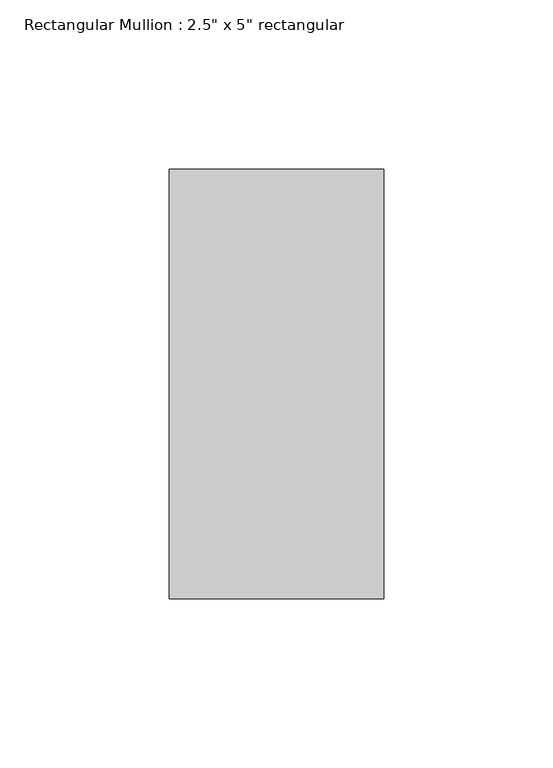
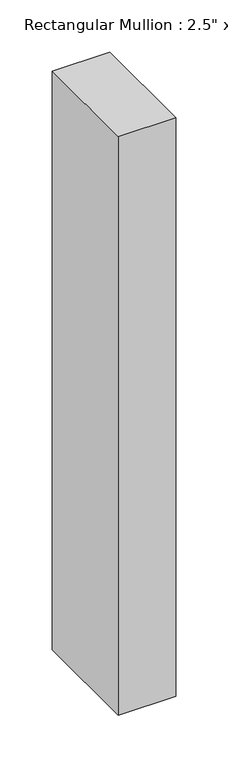
"""IFC4 building model written with IfcOpenShell, lengths in millimetres: member geometry."""

from ifc_helpers import new_model, si_unit, frame, origin, place, context, project, spatial, polyline, outline, extrude, source, transform, mapped, element, save


def member_6428e230(model_context):
    return source(origin(), model_context, "Body", "SweptSolid", [
        extrude(outline(polyline([(31.75, 63.5), (31.75, -63.5), (-31.75, -63.5), (-31.75, 63.5), (31.75, 63.5)])), frame((0.0, 0.0, -677.3333333), z_axis=(0.0, 0.0, 1.0), x_axis=(1.0, 0.0, 0.0)), (0.0, 0.0, 1.0), 677.3333333),
    ])


if __name__ == "__main__":
    model = new_model("IFC4")
    model_context = context("Model", 3, world=origin())
    ifc_project = project(units=[si_unit("LENGTHUNIT", "METRE", prefix="MILLI")], contexts=[model_context])
    site = spatial("IfcSite", under=ifc_project)
    building = spatial("IfcBuilding", under=site)
    placement = place(None, origin())
    member_shape = member_6428e230(model_context)
    element("IfcMember", 1, ObjectType="Rectangular Mullion : 2.5\" x 5\" rectangular", at=placement, inside=building, context=model_context, shape_type="MappedRepresentation", body=[
        mapped(member_shape, transform((0.0, 0.0, 0.0), x_axis=(1.0, 0.0, 0.0), y_axis=(0.0, 1.0, 0.0), z_axis=(0.0, 0.0, 1.0))),
    ])
    save(model, "model.ifc")

# Revit data of these elements
# Type "Rectangular Mullion : 2.5\" x 5\" rectangular"
#   built-in parameter 1007304 = 0.416667 (stored number, unit not read)
#   built-in parameter 1007301 = 0.104167 (stored number, unit not read)
#   built-in parameter 1007300 = 0.104167 (stored number, unit not read)
# Element 1 (IfcMember, "Rectangular Mullion : 2.5\" x 5\" rectangular")
#   Materials on its faces: "door colour"
# Materials
#   "door colour": class "Generic", colour RGB 120 120 120, transparency 0, Cost = 0
